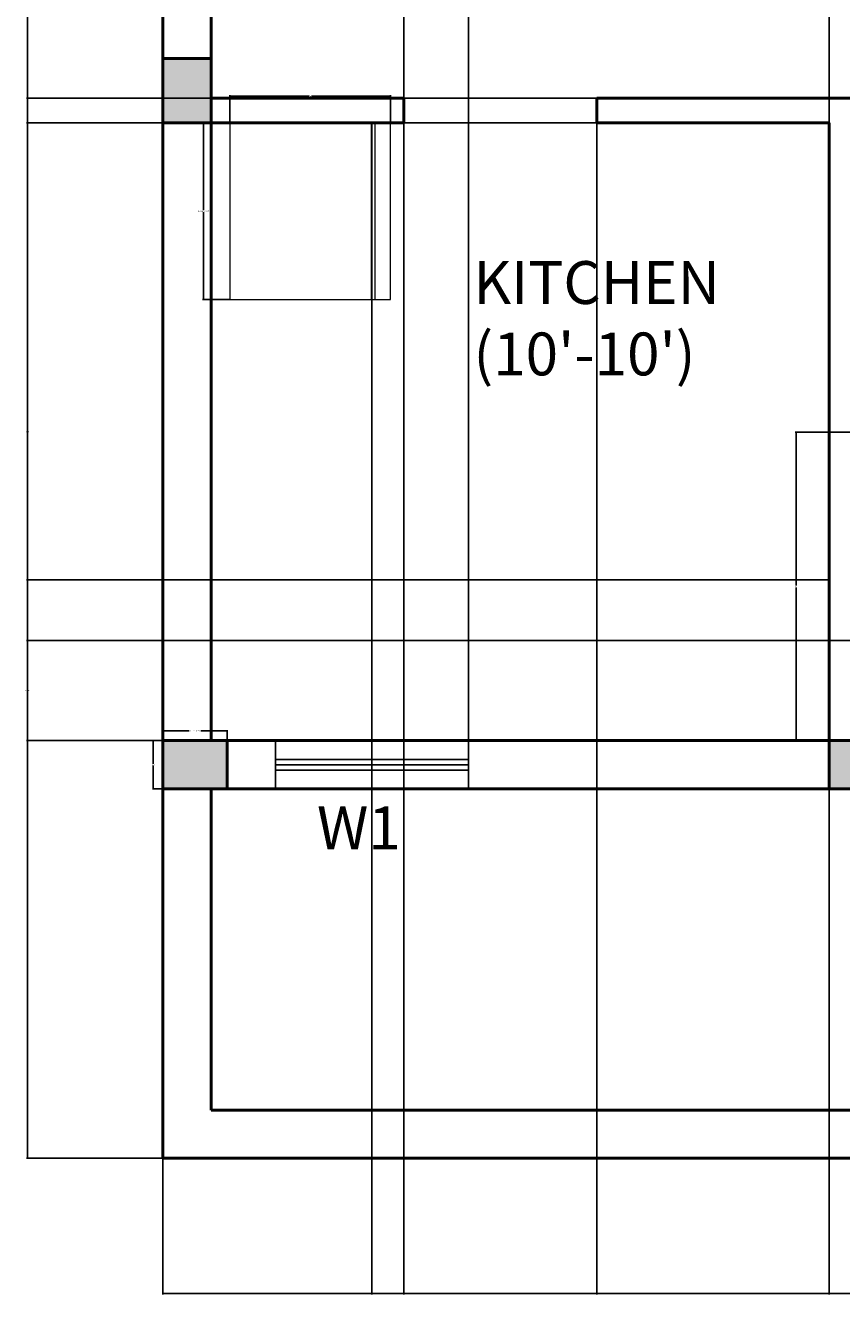
# Model space of a CAD drawing. Units: inches. Extents: x -1517 to -668, y -425 to 52.
# Tile 1 of 13: x -1517 to -1365, y -377 to -140. Entities that reach past the tile are written whole.
import ezdxf

# ---------------------------------------------------------------- set-up
doc = ezdxf.new("R2010")
doc.units = ezdxf.units.IN
doc.header["$MEASUREMENT"] = 0
for name, color, linetype, lineweight in [('A-ANNO-DIMS', 2, 'Continuous', 18), ('A-ANNO-TEXT', 7, 'Continuous', 18), ('A-AREA-IDEN', 7, 'Continuous', 25), ('A-COLS-PATT', 252, 'Continuous', 13), ('A-EQPM', 8, 'Continuous', 18), ('A-FLOR-CASE', 8, 'Continuous', 25), ('column', 7, 'Continuous', 50), ('walls', 240, 'Continuous', 50), ('windows', 140, 'Continuous', 25)]:
    doc.layers.add(name, color=color, linetype=linetype, lineweight=lineweight)
doc.styles.get("Standard").update_dxf_attribs({"font": 'arial.ttf'})
doc.dimstyles.get("Standard").update_dxf_attribs({"dimtxt": 0.18, "dimasz": 0.18, "dimexe": 0.18, "dimexo": 0.0625, "dimgap": 0.09, "dimtad": 0, "dimtih": 1, "dimtoh": 1, "dimdec": 4, "dimzin": 0, "dimdsep": 46, "dimlunit": 4, "dimtxsty": 'Standard', "dimcen": 0.09, "dimadec": 0, "dimazin": 0, "dimtfac": 1, "dimtdec": 4, "dimtofl": 0, "dimtmove": 0, "dimatfit": 3, "dimfxl": 1, "dimtolj": 1, "dimtzin": 0, "dimarcsym": 0})

# ---------------------------------------------------------------- blocks, each defined once
blk = doc.blocks.new('column')
for p, q in [((0, 9), (0, 0)), ((12, 9), (0, 9)), ((12, 0), (12, 9)), ((0, 0), (12, 0))]:
    blk.add_line(p, q)
blk = doc.blocks.new('window 3ft')
for p, q in [((9, 36), (0, 36)), ((3.5, 36), (3.5, 0)), ((4.5, 36), (4.5, 0)), ((5.5, 36), (5.5, 0)), ((9, 0), (0, 0))]:
    blk.add_line(p, q)
blk = doc.blocks.new('REFRIG')
for p, q in [((-0.825, 0.454), (-0.825, -0.454)), ((0, 0.454), (-0.825, 0.454)), ((-0.7462, 0.454), (-0.7462, -0.454)), ((-0.7262, 0.454), (-0.7262, -0.454)), ((0, -0.454), (0, 0.454)), ((-0.825, -0.454), (0, -0.454))]:
    blk.add_line(p, q)
blk = doc.blocks.new('*D16')
at = {"layer": 'A-ANNO-DIMS', "color": 0, "lineweight": -2, "transparency": 16777216}
for p, q in [((-1491.5, -273.31), (-1491.5, -271.39)), ((-1491.32, -271.57), (-1486.61, -271.57)), ((-1479.68, -271.57), (-1484.4, -271.57)), ((-1479.5, -273.31), (-1479.5, -271.39))]:
    blk.add_line(p, q, dxfattribs=at)
at = {"layer": 'A-ANNO-DIMS', "color": 0, "transparency": 16777216}
for points in [[(-1491.32, -271.54), (-1491.32, -271.6), (-1491.5, -271.57)], [(-1479.68, -271.54), (-1479.68, -271.6), (-1479.5, -271.57)]]:
    blk.add_solid(points, dxfattribs=at)
at = {"layer": 'Defpoints', "color": 0, "transparency": 16777216}
for p in [(-1491.5, -271.57), (-1491.5, -273.37), (-1479.5, -273.37)]:
    blk.add_point(p, dxfattribs=at)
at = {"layer": 'A-ANNO-DIMS', "color": 0, "transparency": 16777216, "insert": (-1485.5, -271.57), "char_height": 0.18, "attachment_point": 5}
blk.add_mtext('\\A1;COLUMN 12 TYP.', dxfattribs=at)
blk = doc.blocks.new('*D17')
at = {"layer": 'A-ANNO-DIMS', "color": 0, "lineweight": -2, "transparency": 16777216}
for p, q in [((-1491.57, -273.37), (-1493.48, -273.37)), ((-1493.3, -273.55), (-1493.3, -277.69)), ((-1493.3, -282.19), (-1493.3, -278.05)), ((-1491.57, -282.37), (-1493.48, -282.37))]:
    blk.add_line(p, q, dxfattribs=at)
at = {"layer": 'A-ANNO-DIMS', "color": 0, "transparency": 16777216}
for points in [[(-1493.33, -273.55), (-1493.27, -273.55), (-1493.3, -273.37)], [(-1493.33, -282.19), (-1493.27, -282.19), (-1493.3, -282.37)]]:
    blk.add_solid(points, dxfattribs=at)
at = {"layer": 'Defpoints', "color": 0, "transparency": 16777216}
for p in [(-1491.5, -273.37), (-1493.3, -282.37), (-1491.5, -282.37)]:
    blk.add_point(p, dxfattribs=at)
at = {"layer": 'A-ANNO-DIMS', "color": 0, "transparency": 16777216, "insert": (-1493.3, -277.87), "char_height": 0.18, "attachment_point": 5}
blk.add_mtext('\\A1;9 TYP.', dxfattribs=at)
blk = doc.blocks.new('*D38')
at = {"layer": 'A-ANNO-DIMS', "color": 0, "lineweight": -2, "transparency": 16777216}
for p, q in [((-1479.05, -157.97), (-1484.12, -157.97)), ((-1483.94, -158.15), (-1483.94, -174.3)), ((-1483.94, -190.81), (-1483.94, -174.66)), ((-1479.05, -190.99), (-1484.12, -190.99))]:
    blk.add_line(p, q, dxfattribs=at)
at = {"layer": 'A-ANNO-DIMS', "color": 0, "transparency": 16777216}
for points in [[(-1483.97, -158.15), (-1483.91, -158.15), (-1483.94, -157.97)], [(-1483.97, -190.81), (-1483.91, -190.81), (-1483.94, -190.99)]]:
    blk.add_solid(points, dxfattribs=at)
at = {"layer": 'Defpoints', "color": 0, "transparency": 16777216}
for p in [(-1478.99, -157.97), (-1483.94, -190.99), (-1478.99, -190.99)]:
    blk.add_point(p, dxfattribs=at)
at = {"layer": 'A-ANNO-DIMS', "color": 0, "transparency": 16777216, "insert": (-1483.94, -174.48), "char_height": 0.18, "attachment_point": 5}
blk.add_mtext('\\A1;REFRIGERATOR 33', dxfattribs=at)
blk = doc.blocks.new('*D39')
at = {"layer": 'A-ANNO-DIMS', "color": 0, "lineweight": -2, "transparency": 16777216}
for p, q in [((-1478.99, -157.91), (-1478.99, -152.84)), ((-1478.81, -153.02), (-1464.21, -153.02)), ((-1449.17, -153.02), (-1463.77, -153.02)), ((-1448.99, -157.91), (-1448.99, -152.84))]:
    blk.add_line(p, q, dxfattribs=at)
at = {"layer": 'A-ANNO-DIMS', "color": 0, "transparency": 16777216}
for points in [[(-1478.81, -152.99), (-1478.81, -153.05), (-1478.99, -153.02)], [(-1449.17, -152.99), (-1449.17, -153.05), (-1448.99, -153.02)]]:
    blk.add_solid(points, dxfattribs=at)
at = {"layer": 'Defpoints', "color": 0, "transparency": 16777216}
for p in [(-1478.99, -153.02), (-1478.99, -157.97), (-1448.99, -157.97)]:
    blk.add_point(p, dxfattribs=at)
at = {"layer": 'A-ANNO-DIMS', "color": 0, "transparency": 16777216, "insert": (-1463.99, -153.02), "char_height": 0.18, "attachment_point": 5}
blk.add_mtext('\\A1;30', dxfattribs=at)
blk = doc.blocks.new('*D41')
at = {"layer": 'A-ANNO-DIMS', "color": 0, "lineweight": -2, "transparency": 16777216}
for p, q in [((-1362.57, -215.77), (-1373.48, -215.77)), ((-1373.3, -215.95), (-1373.3, -244.39)), ((-1373.3, -273.19), (-1373.3, -244.75)), ((-1362.57, -273.37), (-1373.48, -273.37))]:
    blk.add_line(p, q, dxfattribs=at)
at = {"layer": 'A-ANNO-DIMS', "color": 0, "transparency": 16777216}
for points in [[(-1373.33, -215.95), (-1373.27, -215.95), (-1373.3, -215.77)], [(-1373.33, -273.19), (-1373.27, -273.19), (-1373.3, -273.37)]]:
    blk.add_solid(points, dxfattribs=at)
at = {"layer": 'Defpoints', "color": 0, "transparency": 16777216}
for p in [(-1362.5, -215.77), (-1373.3, -273.37), (-1362.5, -273.37)]:
    blk.add_point(p, dxfattribs=at)
at = {"layer": 'A-ANNO-DIMS', "color": 0, "transparency": 16777216, "insert": (-1373.3, -244.57), "char_height": 0.18, "attachment_point": 5}
blk.add_mtext('\\A1;58', dxfattribs=at)
blk = doc.blocks.new('*D44')
at = {"layer": 'A-ANNO-DIMS', "color": 0, "lineweight": -2, "transparency": 16777216}
for p, q in [((-1491.5, -351.43), (-1491.5, -376.85)), ((-1005.5, -351.43), (-1005.5, -376.85)), ((-1491.32, -376.67), (-1248.8, -376.67)), ((-1005.68, -376.67), (-1248.21, -376.67))]:
    blk.add_line(p, q, dxfattribs=at)
at = {"layer": 'A-ANNO-DIMS', "color": 0, "transparency": 16777216}
for points in [[(-1491.32, -376.64), (-1491.32, -376.7), (-1491.5, -376.67)], [(-1005.68, -376.64), (-1005.68, -376.7), (-1005.5, -376.67)]]:
    blk.add_solid(points, dxfattribs=at)
at = {"layer": 'Defpoints', "color": 0, "transparency": 16777216}
for p in [(-1491.5, -351.37), (-1005.5, -351.37), (-1005.5, -376.67)]:
    blk.add_point(p, dxfattribs=at)
at = {"layer": 'A-ANNO-DIMS', "color": 0, "transparency": 16777216, "insert": (-1248.5, -376.67), "char_height": 0.18, "attachment_point": 5}
blk.add_mtext('\\A1;486', dxfattribs=at)
blk = doc.blocks.new('*D45')
at = {"layer": 'A-ANNO-DIMS', "color": 0, "lineweight": -2, "transparency": 16777216}
for p, q in [((-1491.57, 26.63), (-1516.98, 26.63)), ((-1516.8, 26.45), (-1516.8, -162.19)), ((-1516.8, -351.19), (-1516.8, -162.55)), ((-1491.57, -351.37), (-1516.98, -351.37))]:
    blk.add_line(p, q, dxfattribs=at)
at = {"layer": 'A-ANNO-DIMS', "color": 0, "transparency": 16777216}
for points in [[(-1516.83, 26.45), (-1516.77, 26.45), (-1516.8, 26.63)], [(-1516.83, -351.19), (-1516.77, -351.19), (-1516.8, -351.37)]]:
    blk.add_solid(points, dxfattribs=at)
at = {"layer": 'Defpoints', "color": 0, "transparency": 16777216}
for p in [(-1491.5, 26.63), (-1516.8, -351.37), (-1491.5, -351.37)]:
    blk.add_point(p, dxfattribs=at)
at = {"layer": 'A-ANNO-DIMS', "color": 0, "transparency": 16777216, "insert": (-1516.8, -162.37), "char_height": 0.18, "attachment_point": 5}
blk.add_mtext('\\A1;378', dxfattribs=at)
blk = doc.blocks.new('*D51')
at = {"layer": 'A-ANNO-DIMS', "color": 0, "lineweight": -2, "transparency": 16777216}
for p, q in [((-1482.5, -273.31), (-1482.5, 52.11)), ((-1482.32, 51.93), (-1425.19, 51.93)), ((-1367.28, 51.93), (-1424.42, 51.93)), ((-1367.1, -273.31), (-1367.1, 52.11))]:
    blk.add_line(p, q, dxfattribs=at)
at = {"layer": 'A-ANNO-DIMS', "color": 0, "transparency": 16777216}
for points in [[(-1482.32, 51.96), (-1482.32, 51.9), (-1482.5, 51.93)], [(-1367.28, 51.96), (-1367.28, 51.9), (-1367.1, 51.93)]]:
    blk.add_solid(points, dxfattribs=at)
at = {"layer": 'Defpoints', "color": 0, "transparency": 16777216}
for p in [(-1367.1, 51.93), (-1482.5, -273.37), (-1367.1, -273.37)]:
    blk.add_point(p, dxfattribs=at)
at = {"layer": 'A-ANNO-DIMS', "color": 0, "transparency": 16777216, "insert": (-1424.8, 51.93), "char_height": 0.18, "attachment_point": 5}
blk.add_mtext('\\A1;115.4', dxfattribs=at)
blk = doc.blocks.new('*D55')
at = {"layer": 'A-ANNO-DIMS', "color": 0, "lineweight": -2, "transparency": 16777216}
for p, q in [((-1482.57, -106.97), (-1516.98, -106.97)), ((-1516.8, -107.15), (-1516.8, -129.99)), ((-1516.8, -153.19), (-1516.8, -130.35)), ((-1482.57, -153.37), (-1516.98, -153.37))]:
    blk.add_line(p, q, dxfattribs=at)
at = {"layer": 'A-ANNO-DIMS', "color": 0, "transparency": 16777216}
for points in [[(-1516.83, -107.15), (-1516.77, -107.15), (-1516.8, -106.97)], [(-1516.83, -153.19), (-1516.77, -153.19), (-1516.8, -153.37)]]:
    blk.add_solid(points, dxfattribs=at)
at = {"layer": 'Defpoints', "color": 0, "transparency": 16777216}
for p in [(-1482.5, -106.97), (-1516.8, -153.37), (-1482.5, -153.37)]:
    blk.add_point(p, dxfattribs=at)
at = {"layer": 'A-ANNO-DIMS', "color": 0, "transparency": 16777216, "insert": (-1516.8, -130.17), "char_height": 0.18, "attachment_point": 5}
blk.add_mtext('\\A1;46.4', dxfattribs=at)
blk = doc.blocks.new('*D56')
at = {"layer": 'A-ANNO-DIMS', "color": 0, "lineweight": -2, "transparency": 16777216}
for p, q in [((-1482.57, -157.97), (-1516.98, -157.97)), ((-1516.8, -158.15), (-1516.8, -215.49)), ((-1516.8, -273.19), (-1516.8, -215.85)), ((-1482.57, -273.37), (-1516.98, -273.37))]:
    blk.add_line(p, q, dxfattribs=at)
at = {"layer": 'A-ANNO-DIMS', "color": 0, "transparency": 16777216}
for points in [[(-1516.83, -158.15), (-1516.77, -158.15), (-1516.8, -157.97)], [(-1516.83, -273.19), (-1516.77, -273.19), (-1516.8, -273.37)]]:
    blk.add_solid(points, dxfattribs=at)
at = {"layer": 'Defpoints', "color": 0, "transparency": 16777216}
for p in [(-1482.5, -157.97), (-1516.8, -273.37), (-1482.5, -273.37)]:
    blk.add_point(p, dxfattribs=at)
at = {"layer": 'A-ANNO-DIMS', "color": 0, "transparency": 16777216, "insert": (-1516.8, -215.67), "char_height": 0.18, "attachment_point": 5}
blk.add_mtext('\\A1;115.4', dxfattribs=at)
blk = doc.blocks.new('*D63')
at = {"layer": 'A-ANNO-DIMS', "color": 0, "lineweight": -2, "transparency": 16777216}
for p, q in [((-1434.48, -282.31), (-1434.48, 52.11)), ((-1434.3, 51.93), (-1401.19, 51.93)), ((-1367.28, 51.93), (-1400.4, 51.93)), ((-1367.1, -282.31), (-1367.1, 52.11))]:
    blk.add_line(p, q, dxfattribs=at)
at = {"layer": 'A-ANNO-DIMS', "color": 0, "transparency": 16777216}
for points in [[(-1434.3, 51.96), (-1434.3, 51.9), (-1434.48, 51.93)], [(-1367.28, 51.96), (-1367.28, 51.9), (-1367.1, 51.93)]]:
    blk.add_solid(points, dxfattribs=at)
at = {"layer": 'Defpoints', "color": 0, "transparency": 16777216}
for p in [(-1367.1, 51.93), (-1434.48, -282.37), (-1367.1, -282.37)]:
    blk.add_point(p, dxfattribs=at)
at = {"layer": 'A-ANNO-DIMS', "color": 0, "transparency": 16777216, "insert": (-1400.79, 51.93), "char_height": 0.18, "attachment_point": 5}
blk.add_mtext('\\A1;67.38', dxfattribs=at)
blk = doc.blocks.new('*D66')
at = {"layer": 'A-ANNO-DIMS', "color": 0, "lineweight": -2, "transparency": 16777216}
for p, q in [((-1014.57, -254.68), (-1516.98, -254.68)), ((-1516.8, -254.86), (-1516.8, -263.85)), ((-1516.8, -273.19), (-1516.8, -264.21)), ((-1014.57, -273.37), (-1516.98, -273.37))]:
    blk.add_line(p, q, dxfattribs=at)
at = {"layer": 'A-ANNO-DIMS', "color": 0, "transparency": 16777216}
for points in [[(-1516.83, -254.86), (-1516.77, -254.86), (-1516.8, -254.68)], [(-1516.83, -273.19), (-1516.77, -273.19), (-1516.8, -273.37)]]:
    blk.add_solid(points, dxfattribs=at)
at = {"layer": 'Defpoints', "color": 0, "transparency": 16777216}
for p in [(-1014.5, -254.68), (-1516.8, -273.37), (-1014.5, -273.37)]:
    blk.add_point(p, dxfattribs=at)
at = {"layer": 'A-ANNO-DIMS', "color": 0, "transparency": 16777216, "insert": (-1516.8, -264.03), "char_height": 0.18, "attachment_point": 5}
blk.add_mtext('\\A1;18.686', dxfattribs=at)
blk = doc.blocks.new('*D67')
at = {"layer": 'A-ANNO-DIMS', "color": 0, "lineweight": -2, "transparency": 16777216}
for p, q in [((-1482.5, -157.91), (-1482.5, 52.11)), ((-1482.32, 51.93), (-1464.72, 51.93)), ((-1446.68, 51.93), (-1464.28, 51.93)), ((-1446.5, -157.91), (-1446.5, 52.11))]:
    blk.add_line(p, q, dxfattribs=at)
at = {"layer": 'A-ANNO-DIMS', "color": 0, "transparency": 16777216}
for points in [[(-1482.32, 51.96), (-1482.32, 51.9), (-1482.5, 51.93)], [(-1446.68, 51.96), (-1446.68, 51.9), (-1446.5, 51.93)]]:
    blk.add_solid(points, dxfattribs=at)
at = {"layer": 'Defpoints', "color": 0, "transparency": 16777216}
for p in [(-1446.5, 51.93), (-1482.5, -157.97), (-1446.5, -157.97)]:
    blk.add_point(p, dxfattribs=at)
at = {"layer": 'A-ANNO-DIMS', "color": 0, "transparency": 16777216, "insert": (-1464.5, 51.93), "char_height": 0.18, "attachment_point": 5}
blk.add_mtext('\\A1;36', dxfattribs=at)
blk = doc.blocks.new('*D68')
at = {"layer": 'A-ANNO-DIMS', "color": 0, "lineweight": -2, "transparency": 16777216}
for p, q in [((-1446.5, -158.03), (-1446.5, -376.85)), ((-1410.5, -158.03), (-1410.5, -376.85)), ((-1446.32, -376.67), (-1428.72, -376.67)), ((-1410.68, -376.67), (-1428.28, -376.67))]:
    blk.add_line(p, q, dxfattribs=at)
at = {"layer": 'A-ANNO-DIMS', "color": 0, "transparency": 16777216}
for points in [[(-1446.32, -376.64), (-1446.32, -376.7), (-1446.5, -376.67)], [(-1410.68, -376.64), (-1410.68, -376.7), (-1410.5, -376.67)]]:
    blk.add_solid(points, dxfattribs=at)
at = {"layer": 'Defpoints', "color": 0, "transparency": 16777216}
for p in [(-1446.5, -157.97), (-1410.5, -157.97), (-1410.5, -376.67)]:
    blk.add_point(p, dxfattribs=at)
at = {"layer": 'A-ANNO-DIMS', "color": 0, "transparency": 16777216, "insert": (-1428.5, -376.67), "char_height": 0.18, "attachment_point": 5}
blk.add_mtext('\\A1;36', dxfattribs=at)
blk = doc.blocks.new('*D74')
at = {"layer": 'A-ANNO-DIMS', "color": 0, "lineweight": -2, "transparency": 16777216}
for p, q in [((-1452.5, -243.43), (-1452.5, -376.85)), ((-1367.1, -243.43), (-1367.1, -376.85)), ((-1452.32, -376.67), (-1410.13, -376.67)), ((-1367.28, -376.67), (-1409.48, -376.67))]:
    blk.add_line(p, q, dxfattribs=at)
at = {"layer": 'A-ANNO-DIMS', "color": 0, "transparency": 16777216}
for points in [[(-1452.32, -376.64), (-1452.32, -376.7), (-1452.5, -376.67)], [(-1367.28, -376.64), (-1367.28, -376.7), (-1367.1, -376.67)]]:
    blk.add_solid(points, dxfattribs=at)
at = {"layer": 'Defpoints', "color": 0, "transparency": 16777216}
for p in [(-1452.5, -243.37), (-1367.1, -243.37), (-1367.1, -376.67)]:
    blk.add_point(p, dxfattribs=at)
at = {"layer": 'A-ANNO-DIMS', "color": 0, "transparency": 16777216, "insert": (-1409.8, -376.67), "char_height": 0.18, "attachment_point": 5}
blk.add_mtext('\\A1;85.4', dxfattribs=at)
blk = doc.blocks.new('*D75')
at = {"layer": 'A-ANNO-DIMS', "color": 0, "lineweight": -2, "transparency": 16777216}
for p, q in [((-1452.57, -243.37), (-1516.98, -243.37)), ((-1516.8, -243.55), (-1516.8, -258.19)), ((-1516.8, -273.19), (-1516.8, -258.55)), ((-1434.54, -273.37), (-1516.98, -273.37))]:
    blk.add_line(p, q, dxfattribs=at)
at = {"layer": 'A-ANNO-DIMS', "color": 0, "transparency": 16777216}
for points in [[(-1516.83, -243.55), (-1516.77, -243.55), (-1516.8, -243.37)], [(-1516.83, -273.19), (-1516.77, -273.19), (-1516.8, -273.37)]]:
    blk.add_solid(points, dxfattribs=at)
at = {"layer": 'Defpoints', "color": 0, "transparency": 16777216}
for p in [(-1452.5, -243.37), (-1516.8, -273.37), (-1434.48, -273.37)]:
    blk.add_point(p, dxfattribs=at)
at = {"layer": 'A-ANNO-DIMS', "color": 0, "transparency": 16777216, "insert": (-1516.8, -258.37), "char_height": 0.18, "attachment_point": 5}
blk.add_mtext('\\A1;30', dxfattribs=at)
blk = doc.blocks.new('*D76')
at = {"layer": 'A-ANNO-DIMS', "color": 0, "lineweight": -2, "transparency": 16777216}
for p, q in [((-1410.57, -153.37), (-1516.98, -153.37)), ((-1516.8, -153.55), (-1516.8, -155.49)), ((-1516.8, -157.79), (-1516.8, -155.85)), ((-1410.57, -157.97), (-1516.98, -157.97))]:
    blk.add_line(p, q, dxfattribs=at)
at = {"layer": 'A-ANNO-DIMS', "color": 0, "transparency": 16777216}
for points in [[(-1516.83, -153.55), (-1516.77, -153.55), (-1516.8, -153.37)], [(-1516.83, -157.79), (-1516.77, -157.79), (-1516.8, -157.97)]]:
    blk.add_solid(points, dxfattribs=at)
at = {"layer": 'Defpoints', "color": 0, "transparency": 16777216}
for p in [(-1516.8, -153.37), (-1410.5, -153.37), (-1410.5, -157.97)]:
    blk.add_point(p, dxfattribs=at)
at = {"layer": 'A-ANNO-DIMS', "color": 0, "transparency": 16777216, "insert": (-1516.8, -155.67), "char_height": 0.18, "attachment_point": 5}
blk.add_mtext('\\A1;4.6', dxfattribs=at)

msp = doc.modelspace()

# ---------------------------------------------------------------- hatches: boundary and pattern name
at = {"layer": 'A-COLS-PATT'}
h = msp.add_hatch(dxfattribs=at)
h.set_pattern_fill('AR-CONC', color=256, scale=0.69)
h.set_pattern_definition([(50, (0, 0), (4.949095, -0.43299), [0.5175, -5.6925]), (355, (0, 0), (-0.957384, 5.190126), [0.414, -4.554]), (100.45144, (0.4124, -0.036), (3.991711, 4.757136), [0.439807, -4.83788]), (46.1842, (0, 1.38), (7.363965, -1.142083), [0.77625, -8.53875]), (96.63564, (0.614, 1.285), (6.449167, 6.72142), [0.65971, -7.256825]), (351.18416, (0, 1.38), (6.449167, 6.72142), [0.621, -6.831]), (21, (0.69, 1.035), (4.118659, -2.77807), [0.5175, -5.6925]), (326, (0.69, 1.035), (1.678876, 5.003535), [0.414, -4.554]), (71.45144, (1.033, 0.8035), (5.797534, 2.225465), [0.439807, -4.83788]), (37.5, (0, 0), (0.083903, 2.2969676), [0, -4.4988, 0, -4.623, 0, -4.57125]), (7.5, (0, 0), (1.81518, 2.721441), [0, -2.6358, 0, -4.3953, 0, -1.74225]), (327.5, (-1.5387, 0), (3.6833748, -0.1556286), [0, -1.725, 0, -5.382, 0, -7.1415]), (317.5, (-2.2287, 0), (4.0239846, 0.6907244), [0, -2.2425, 0, -3.5742, 0, -5.0715])])
h.paths.add_polyline_path([(-1491.5037, 26.63), (-1491.5037, 17.63), (-1479.5037, 17.63), (-1479.5037, 26.63)])
h.paths.add_polyline_path([(-1278.5037, 17.63), (-1278.5037, 26.63), (-1290.5037, 26.63), (-1290.5037, 17.63)])
h.paths.add_polyline_path([(-1177.9037, 26.63), (-1189.9037, 26.63), (-1189.9037, 17.63), (-1177.9037, 17.63)])
h.paths.add_polyline_path([(-1017.5037, 26.63), (-1017.5037, 17.63), (-1005.5037, 17.63), (-1005.5037, 26.63)])
h.paths.add_polyline_path([(-1005.5037, -270.37), (-1014.5037, -270.37), (-1014.5037, -282.37), (-1005.5037, -282.37)])
h.paths.add_polyline_path([(-1247.1037, -282.37), (-1235.1037, -282.37), (-1235.1037, -273.37), (-1247.1037, -273.37)])
h.paths.add_polyline_path([(-1367.1037, -273.37), (-1367.1037, -282.37), (-1355.1037, -282.37), (-1355.1037, -273.37)])
h.paths.add_polyline_path([(-1491.5037, -282.37), (-1479.5037, -282.37), (-1479.5037, -273.37), (-1491.5037, -273.37)])
h.paths.add_polyline_path([(-1482.5037, -145.97), (-1491.5037, -145.97), (-1491.5037, -157.97), (-1482.5037, -157.97)])
h.paths.add_polyline_path([(-1491.5037, -94.97), (-1491.5037, -106.97), (-1482.5037, -106.97), (-1482.5037, -94.97)])

# ---------------------------------------------------------------- linework, layer by layer
at = {"layer": 'A-FLOR-CASE'}
for q in [(-1452.5037, -157.97), (-1367.1037, -243.37)]:
    msp.add_line((-1452.5037, -243.37), q, dxfattribs=at)
at = {"layer": 'walls'}
for p, q in [((-1491.5037, 26.63), (-1491.5037, -351.37)), ((-1482.5037, -106.97), (-1482.5037, -153.37)), ((-1482.5037, -153.37), (-1446.5037, -153.37)), ((-1446.5037, -157.97), (-1446.5037, -153.37)), ((-1410.5037, -157.97), (-1410.5037, -153.37)), ((-1410.5037, -153.37), (-1362.5037, -153.37)), ((-1482.5037, -273.37), (-1482.5037, -157.97)), ((-1482.5037, -157.97), (-1446.5037, -157.97)), ((-1482.5037, -157.97), (-1446.5037, -157.97)), ((-1482.5037, -157.97), (-1482.5037, -273.37)), ((-1410.5037, -157.97), (-1367.1037, -157.97)), ((-1367.1037, -157.97), (-1367.1037, -273.37)), ((-1482.5037, -273.37), (-1367.1037, -273.37)), ((-1482.5037, -282.37), (-1114.0183, -282.37)), ((-1482.5037, -282.37), (-1482.5037, -342.37)), ((-1482.5037, -342.37), (-1014.5037, -342.37)), ((-1491.5037, -351.37), (-1005.5037, -351.37))]:
    msp.add_line(p, q, dxfattribs=at)

# ---------------------------------------------------------------- block references
at = {"layer": 'A-EQPM', "xscale": 36.36363636367646, "yscale": 36.36363636367646, "zscale": 36.36363636367646, "rotation": 180}
msp.add_blockref('REFRIG', (-1478.992, -174.4791), dxfattribs=at)
at = {"layer": 'column'}
for p, rotation in [((-1491.5037, -145.97), 270), ((-1479.5037, -273.37), 180), ((-1355.1037, -273.37), 180)]:
    msp.add_blockref('column', p, dxfattribs=dict(at, rotation=rotation))
at = {"layer": 'windows', "rotation": 270}
msp.add_blockref('window 3ft', (-1470.4795, -273.37), dxfattribs=at)

# ---------------------------------------------------------------- texts
at = {"layer": 'A-ANNO-TEXT', "insert": (-1462.7437, -285.6776), "char_height": 8, "attachment_point": 1}
msp.add_mtext_dynamic_manual_height_columns('{\\fArial|b1|i0|c0|p34;W1}', width=23.131632, gutter_width=1, heights=[0], dxfattribs=at)
at = {"layer": 'A-AREA-IDEN', "insert": (-1433.5354, -183.8139), "char_height": 8, "attachment_point": 1}
msp.add_mtext_dynamic_manual_height_columns("{\\fArial|b1|i0|c0|p34;KITCHEN\\P(10'-10')}", width=59.221472, gutter_width=1, heights=[0], dxfattribs=at)

# ---------------------------------------------------------------- dimensions: what is measured, and where the dimension line sits
at = {"layer": 'A-ANNO-DIMS'}
for base, p1, p2, override, picture, middle in [((-1367.1037, 51.93), (-1482.5037, -273.37), (-1367.1037, -273.37), {"dimdec": 1, "dimlfac": 1, "dimrnd": 0, "dimzin": 0, "dimdsep": 46, "dimlunit": 2}, '*D51', (-1424.8037, 51.93)), ((-1446.5037, 51.93), (-1482.5037, -157.97), (-1446.5037, -157.97), {"dimdec": 0, "dimlfac": 1, "dimrnd": 0, "dimzin": 0, "dimdsep": 46, "dimlunit": 2}, '*D67', (-1464.5037, 51.93)), ((-1367.1037, 51.93), (-1434.4795, -282.37), (-1367.1037, -282.37), {"dimdec": 2, "dimlfac": 1, "dimrnd": 0, "dimzin": 0, "dimdsep": 46, "dimlunit": 2}, '*D63', (-1400.7916, 51.93)), ((-1410.5037, -376.67), (-1446.5037, -157.97), (-1410.5037, -157.97), {"dimdec": 0, "dimlfac": 1, "dimrnd": 0, "dimzin": 0, "dimdsep": 46, "dimlunit": 2}, '*D68', (-1428.5037, -376.67)), ((-1367.1037, -376.67), (-1452.5037, -243.37), (-1367.1037, -243.37), {"dimdec": 1, "dimlfac": 1, "dimrnd": 0, "dimzin": 0, "dimdsep": 46, "dimlunit": 2}, '*D74', (-1409.8037, -376.67)), ((-1005.5037, -376.67), (-1491.5037, -351.37), (-1005.5037, -351.37), {"dimdec": 0, "dimlfac": 1, "dimrnd": 0, "dimzin": 0, "dimdsep": 46, "dimlunit": 2}, '*D44', (-1248.5037, -376.67))]:
    dim = msp.add_linear_dim(base=base, p1=p1, p2=p2, dimstyle='Standard', override=override, dxfattribs=at)
    dim.commit()
    dim.dimension.update_dxf_attribs({"geometry": picture, "text_midpoint": middle})
for base, p1, p2, angle, override, picture, middle in [((-1516.8037, -351.37), (-1491.5037, 26.63), (-1491.5037, -351.37), 90, {"dimdec": 0, "dimlfac": 1, "dimrnd": 0, "dimzin": 0, "dimdsep": 46, "dimlunit": 2}, '*D45', (-1516.8037, -162.37)), ((-1516.8037, -153.37), (-1482.5037, -106.97), (-1482.5037, -153.37), 90, {"dimdec": 1, "dimlfac": 1, "dimrnd": 0, "dimzin": 0, "dimdsep": 46, "dimlunit": 2}, '*D55', (-1516.8037, -130.17)), ((-1516.8037, -153.37), (-1410.5037, -157.97), (-1410.5037, -153.37), 90, {"dimdec": 1, "dimlfac": 1, "dimrnd": 0, "dimzin": 0, "dimdsep": 46, "dimlunit": 2}, '*D76', (-1516.8037, -155.67)), ((-1478.992, -153.0173), (-1448.992, -157.97), (-1478.992, -157.97), 180, {"dimdec": 0, "dimlfac": 1, "dimrnd": 0, "dimzin": 0, "dimdsep": 46, "dimlunit": 2}, '*D39', (-1463.992, -153.0173)), ((-1516.8037, -273.37), (-1482.5037, -157.97), (-1482.5037, -273.37), 90, {"dimdec": 1, "dimlfac": 1, "dimrnd": 0, "dimzin": 0, "dimdsep": 46, "dimlunit": 2}, '*D56', (-1516.8037, -215.67)), ((-1373.3037, -273.37), (-1362.5037, -215.77), (-1362.5037, -273.37), 270, {"dimdec": 0, "dimlfac": 1, "dimrnd": 0, "dimzin": 0, "dimdsep": 46, "dimlunit": 2}, '*D41', (-1373.3037, -244.57)), ((-1516.8037, -273.37), (-1452.5037, -243.37), (-1434.4795, -273.37), 90, {"dimdec": 0, "dimlfac": 1, "dimrnd": 0, "dimzin": 0, "dimdsep": 46, "dimlunit": 2}, '*D75', (-1516.8037, -258.37)), ((-1516.8037, -273.37), (-1014.5037, -254.6839), (-1014.5037, -273.37), 90, {"dimdec": 3, "dimlfac": 1, "dimrnd": 0, "dimzin": 0, "dimdsep": 46, "dimlunit": 2}, '*D66', (-1516.8037, -264.0269))]:
    dim = msp.add_linear_dim(base=base, p1=p1, p2=p2, angle=angle, dimstyle='Standard', override=override, dxfattribs=at)
    dim.commit()
    dim.dimension.update_dxf_attribs({"geometry": picture, "text_midpoint": middle})
for base, p1, p2, angle, text, picture, middle in [((-1483.9447, -190.9882), (-1478.992, -157.97), (-1478.992, -190.9882), 270, 'REFRIGERATOR <>', '*D38', (-1483.9447, -174.4791)), ((-1491.5037, -271.57), (-1479.5037, -273.37), (-1491.5037, -273.37), 180, 'COLUMN <> TYP.', '*D16', (-1485.5037, -271.57)), ((-1493.3037, -282.37), (-1491.5037, -273.37), (-1491.5037, -282.37), 270, '<> TYP.', '*D17', (-1493.3037, -277.87))]:
    dim = msp.add_linear_dim(base=base, p1=p1, p2=p2, angle=angle, text=text, dimstyle='Standard', override={"dimdec": 0, "dimlfac": 1, "dimrnd": 0, "dimzin": 0, "dimdsep": 46, "dimlunit": 2}, dxfattribs=at)
    dim.commit()
    dim.dimension.update_dxf_attribs({"geometry": picture, "text_midpoint": middle})

doc.saveas('drawing.dxf')
